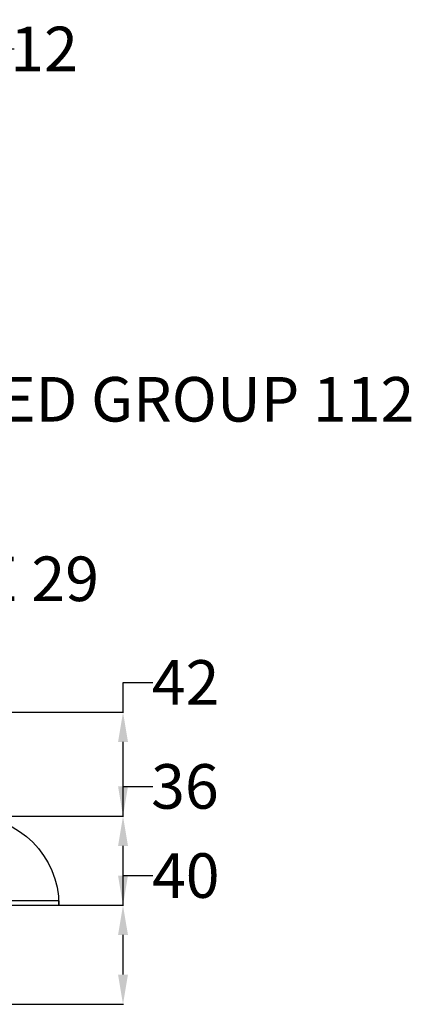
# Model space of a CAD drawing. Units: inches. Extents: x -478 to 256, y -93 to 343.
# Tile 5 of 5: x 98 to 256, y -55 to 343. Entities that reach past the tile are written whole.
import ezdxf

# ---------------------------------------------------------------- set-up
doc = ezdxf.new("R2010")
doc.units = ezdxf.units.IN
doc.layers.add('A-ANNO-DIMS', color=2, linetype='Continuous', lineweight=18)
doc.layers.add('A-DOOR', color=3, linetype='Continuous', lineweight=25)
doc.styles.get("Standard").update_dxf_attribs({"font": 'arial.ttf'})
doc.dimstyles.get("Standard").update_dxf_attribs({"dimtxt": 18, "dimasz": 12, "dimexe": 0.18, "dimexo": 0.0625, "dimgap": 0.09, "dimtad": 0, "dimtih": 1, "dimtoh": 1, "dimdec": 0, "dimzin": 0, "dimdsep": 46, "dimlunit": 3, "dimtxsty": 'Standard', "dimcen": 0.09, "dimadec": 0, "dimazin": 0, "dimtfac": 1, "dimtdec": 0, "dimtofl": 0, "dimtmove": 0, "dimatfit": 3, "dimfxl": 1, "dimtolj": 1, "dimtzin": 0, "dimarcsym": 0})

# ---------------------------------------------------------------- blocks, each defined once
blk = doc.blocks.new('*U14')
for p, q in [((0, 0), (0, -6)), ((36, 0), (36, -6))]:
    blk.add_line(p, q)
blk.add_lwpolyline([(0, 0), (0, 36), (1.75, 36), (1.75, 0)], close=True)
blk.add_arc((0, 0), 36, 0, 90)
blk = doc.blocks.new('*D17')
at = {"layer": 'A-ANNO-DIMS', "color": 0, "lineweight": -2, "transparency": 16777216}
for p, q in [((-32.43, 120.92), (-32.43, 116.52)), ((-3.86, 120.92), (-3.86, 116.52)), ((-20.43, 116.7), (-15.86, 116.7)), ((-3.86, 116.7), (8.14, 116.7))]:
    blk.add_line(p, q, dxfattribs=at)
at = {"layer": 'A-ANNO-DIMS', "color": 0, "transparency": 16777216}
for points in [[(-20.43, 118.7), (-20.43, 114.7), (-32.43, 116.7)], [(-15.86, 118.7), (-15.86, 114.7), (-3.86, 116.7)]]:
    blk.add_solid(points, dxfattribs=at)
at = {"layer": 'Defpoints', "color": 0, "transparency": 16777216}
for p in [(-32.43, 120.98), (-3.86, 120.98), (-3.86, 116.7)]:
    blk.add_point(p, dxfattribs=at)
at = {"layer": 'A-ANNO-DIMS', "color": 0, "transparency": 16777216, "insert": (71.63, 116.7), "char_height": 18, "attachment_point": 5}
blk.add_mtext('\\A1;FRIDGE 29', dxfattribs=at)
blk = doc.blocks.new('*D27')
at = {"layer": 'A-ANNO-DIMS', "color": 0, "lineweight": -2, "transparency": 16777216}
for p, q in [((-56.12, 205.87), (-56.12, 189.02)), ((55.39, 205.87), (55.39, 189.02)), ((-44.12, 189.2), (43.39, 189.2)), ((55.39, 189.2), (67.39, 189.2))]:
    blk.add_line(p, q, dxfattribs=at)
at = {"layer": 'A-ANNO-DIMS', "color": 0, "transparency": 16777216}
for points in [[(-44.12, 191.2), (-44.12, 187.2), (-56.12, 189.2)], [(43.39, 191.2), (43.39, 187.2), (55.39, 189.2)]]:
    blk.add_solid(points, dxfattribs=at)
at = {"layer": 'Defpoints', "color": 0, "transparency": 16777216}
for p in [(-56.12, 205.93), (55.39, 205.93), (55.39, 189.2)]:
    blk.add_point(p, dxfattribs=at)
at = {"layer": 'A-ANNO-DIMS', "color": 0, "transparency": 16777216, "insert": (165.82, 189.2), "char_height": 18, "attachment_point": 5}
blk.add_mtext('\\A1;BED GROUP 112', dxfattribs=at)
blk = doc.blocks.new('*D39')
at = {"layer": 'A-ANNO-DIMS', "color": 0, "lineweight": -2, "transparency": 16777216}
for p, q in [((140.01, -15.16), (140.01, -3.16)), ((140.01, -3.16), (152.01, -3.16)), ((78.21, -15.16), (140.19, -15.16)), ((140.01, -43.16), (140.01, -27.16)), ((78.21, -55.16), (140.19, -55.16))]:
    blk.add_line(p, q, dxfattribs=at)
at = {"layer": 'A-ANNO-DIMS', "color": 0, "transparency": 16777216}
for points in [[(138.01, -27.16), (142.01, -27.16), (140.01, -15.16)], [(138.01, -43.16), (142.01, -43.16), (140.01, -55.16)]]:
    blk.add_solid(points, dxfattribs=at)
at = {"layer": 'Defpoints', "color": 0, "transparency": 16777216}
for p in [(78.14, -15.16), (140.01, -15.16), (78.14, -55.16)]:
    blk.add_point(p, dxfattribs=at)
at = {"layer": 'A-ANNO-DIMS', "color": 0, "transparency": 16777216, "insert": (165.32, -3.16), "char_height": 18, "attachment_point": 5}
blk.add_mtext('\\A1;40', dxfattribs=at)
blk = doc.blocks.new('*D40')
at = {"layer": 'A-ANNO-DIMS', "color": 0, "lineweight": -2, "transparency": 16777216}
for p, q in [((140.01, 20.84), (140.01, 32.84)), ((140.01, 32.84), (152.01, 32.84)), ((78.21, 20.84), (140.19, 20.84)), ((140.01, -3.16), (140.01, 8.84)), ((78.21, -15.16), (140.19, -15.16))]:
    blk.add_line(p, q, dxfattribs=at)
at = {"layer": 'A-ANNO-DIMS', "color": 0, "transparency": 16777216}
for points in [[(138.01, 8.84), (142.01, 8.84), (140.01, 20.84)], [(138.01, -3.16), (142.01, -3.16), (140.01, -15.16)]]:
    blk.add_solid(points, dxfattribs=at)
at = {"layer": 'Defpoints', "color": 0, "transparency": 16777216}
for p in [(78.14, 20.84), (140.01, 20.84), (78.14, -15.16)]:
    blk.add_point(p, dxfattribs=at)
at = {"layer": 'A-ANNO-DIMS', "color": 0, "transparency": 16777216, "insert": (164.98, 32.84), "char_height": 18, "attachment_point": 5}
blk.add_mtext('\\A1;36', dxfattribs=at)
blk = doc.blocks.new('*D41')
at = {"layer": 'A-ANNO-DIMS', "color": 0, "lineweight": -2, "transparency": 16777216}
for p, q in [((140.01, 62.84), (140.01, 74.84)), ((140.01, 74.84), (152.01, 74.84)), ((72.21, 62.84), (140.19, 62.84)), ((140.01, 32.84), (140.01, 50.84)), ((78.21, 20.84), (140.19, 20.84))]:
    blk.add_line(p, q, dxfattribs=at)
at = {"layer": 'A-ANNO-DIMS', "color": 0, "transparency": 16777216}
for points in [[(138.01, 50.84), (142.01, 50.84), (140.01, 62.84)], [(138.01, 32.84), (142.01, 32.84), (140.01, 20.84)]]:
    blk.add_solid(points, dxfattribs=at)
at = {"layer": 'Defpoints', "color": 0, "transparency": 16777216}
for p in [(72.14, 62.84), (140.01, 62.84), (78.14, 20.84)]:
    blk.add_point(p, dxfattribs=at)
at = {"layer": 'A-ANNO-DIMS', "color": 0, "transparency": 16777216, "insert": (165.26, 74.84), "char_height": 18, "attachment_point": 5}
blk.add_mtext('\\A1;42', dxfattribs=at)
blk = doc.blocks.new('*D51')
at = {"layer": 'A-ANNO-DIMS', "color": 0, "lineweight": -2, "transparency": 16777216}
for p, q in [((48.14, 330.71), (36.14, 330.71)), ((60.14, 154.9), (60.14, 330.89)), ((72.14, 154.9), (72.14, 330.89)), ((84.14, 330.71), (96.14, 330.71))]:
    blk.add_line(p, q, dxfattribs=at)
at = {"layer": 'A-ANNO-DIMS', "color": 0, "transparency": 16777216}
for points in [[(48.14, 332.71), (48.14, 328.71), (60.14, 330.71)], [(84.14, 332.71), (84.14, 328.71), (72.14, 330.71)]]:
    blk.add_solid(points, dxfattribs=at)
at = {"layer": 'Defpoints', "color": 0, "transparency": 16777216}
for p in [(72.14, 330.71), (60.14, 154.84), (72.14, 154.84)]:
    blk.add_point(p, dxfattribs=at)
at = {"layer": 'A-ANNO-DIMS', "color": 0, "transparency": 16777216, "insert": (108.19, 330.71), "char_height": 18, "attachment_point": 5}
blk.add_mtext('\\A1;12', dxfattribs=at)

msp = doc.modelspace()

# ---------------------------------------------------------------- block references
at = {"layer": 'A-DOOR', "xscale": -1, "rotation": 270}
msp.add_blockref('*U14', (78.144, -15.159), dxfattribs=at)

# ---------------------------------------------------------------- dimensions: what is measured, and where the dimension line sits
at = {"layer": 'A-ANNO-DIMS'}
dim = msp.add_linear_dim(base=(72.144, 330.706), p1=(60.144, 154.841), p2=(72.144, 154.841), dimstyle='Standard', override={"dimdec": 0, "dimlfac": 1, "dimrnd": 0, "dimzin": 0, "dimdsep": 46, "dimlunit": 2}, dxfattribs=at)
dim.commit()
dim.dimension.update_dxf_attribs({"geometry": '*D51', "text_midpoint": (108.187, 330.706)})
for base, p1, p2, text, picture, middle in [((55.394, 189.204), (-56.116, 205.93), (55.394, 205.93), 'BED GROUP <>', '*D27', (165.821, 189.204)), ((-3.856, 116.697), (-32.426, 120.982), (-3.856, 120.982), 'FRIDGE <>', '*D17', (71.627, 116.697))]:
    dim = msp.add_linear_dim(base=base, p1=p1, p2=p2, text=text, dimstyle='Standard', override={"dimdec": 0, "dimlfac": 1, "dimrnd": 0, "dimzin": 0, "dimdsep": 46, "dimlunit": 2}, dxfattribs=at)
    dim.commit()
    dim.dimension.update_dxf_attribs({"geometry": picture, "text_midpoint": middle})
for base, p1, p2, picture, middle in [((140.009, 62.841), (78.144, 20.841), (72.144, 62.841), '*D41', (165.262, 74.841)), ((140.009, 20.841), (78.144, -15.159), (78.144, 20.841), '*D40', (164.979, 32.841)), ((140.009, -15.159), (78.144, -55.159), (78.144, -15.159), '*D39', (165.323, -3.159))]:
    dim = msp.add_linear_dim(base=base, p1=p1, p2=p2, angle=90, dimstyle='Standard', override={"dimdec": 0, "dimlfac": 1, "dimrnd": 0, "dimzin": 0, "dimdsep": 46, "dimlunit": 2}, dxfattribs=at)
    dim.commit()
    dim.dimension.update_dxf_attribs({"geometry": picture, "text_midpoint": middle})

doc.saveas('drawing.dxf')
